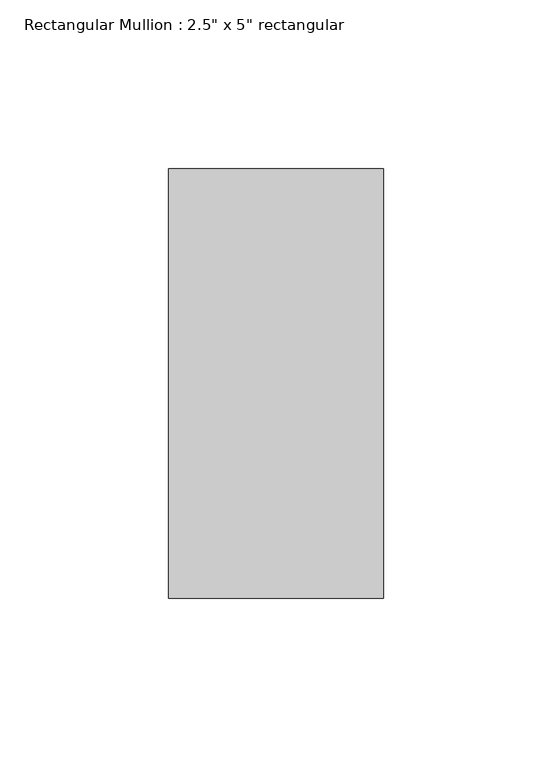
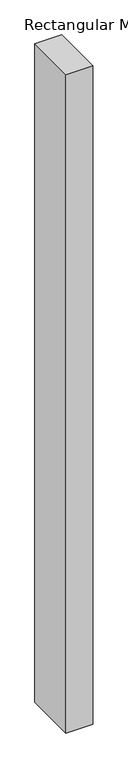
"""IFC4 building model written with IfcOpenShell, lengths in millimetres: member geometry."""

from ifc_helpers import new_model, si_unit, frame, origin, place, context, project, spatial, polyline, outline, extrude, source, transform, mapped, element, save


def member_fad113ab(model_context):
    return source(origin(), model_context, "Body", "SweptSolid", [
        extrude(outline(polyline([(31.75, 63.5), (31.75, -63.5), (-31.75, -63.5), (-31.75, 63.5), (31.75, 63.5)])), frame((0.0, 0.0, -1646.9538703), z_axis=(0.0, 0.0, 1.0), x_axis=(1.0, 0.0, 0.0)), (0.0, 0.0, 1.0), 1646.9538703),
    ])


if __name__ == "__main__":
    model = new_model("IFC4")
    model_context = context("Model", 3, world=origin())
    ifc_project = project(units=[si_unit("LENGTHUNIT", "METRE", prefix="MILLI")], contexts=[model_context])
    site = spatial("IfcSite", under=ifc_project)
    building = spatial("IfcBuilding", under=site)
    placement = place(None, origin())
    member_shape = member_fad113ab(model_context)
    element("IfcMember", 1, ObjectType="Rectangular Mullion : 2.5\" x 5\" rectangular", at=placement, inside=building, context=model_context, shape_type="MappedRepresentation", body=[
        mapped(member_shape, transform((0.0, 0.0, 0.0), x_axis=(1.0, 0.0, 0.0), y_axis=(0.0, 1.0, 0.0), z_axis=(0.0, 0.0, 1.0))),
    ])
    save(model, "model.ifc")

# Revit data of these elements
# Type "Rectangular Mullion : 2.5\" x 5\" rectangular"
#   built-in parameter 1007304 = 0.416667 (stored number, unit not read)
#   built-in parameter 1007301 = 0.104167 (stored number, unit not read)
#   built-in parameter 1007300 = 0.104167 (stored number, unit not read)
# Element 1 (IfcMember, "Rectangular Mullion : 2.5\" x 5\" rectangular")
#   Materials on its faces: "Aluminum"
# Materials
#   "Aluminum": class "Metal", colour RGB 247 247 247, transparency 0, Description = "Aluminum 6061", Cost = 0
